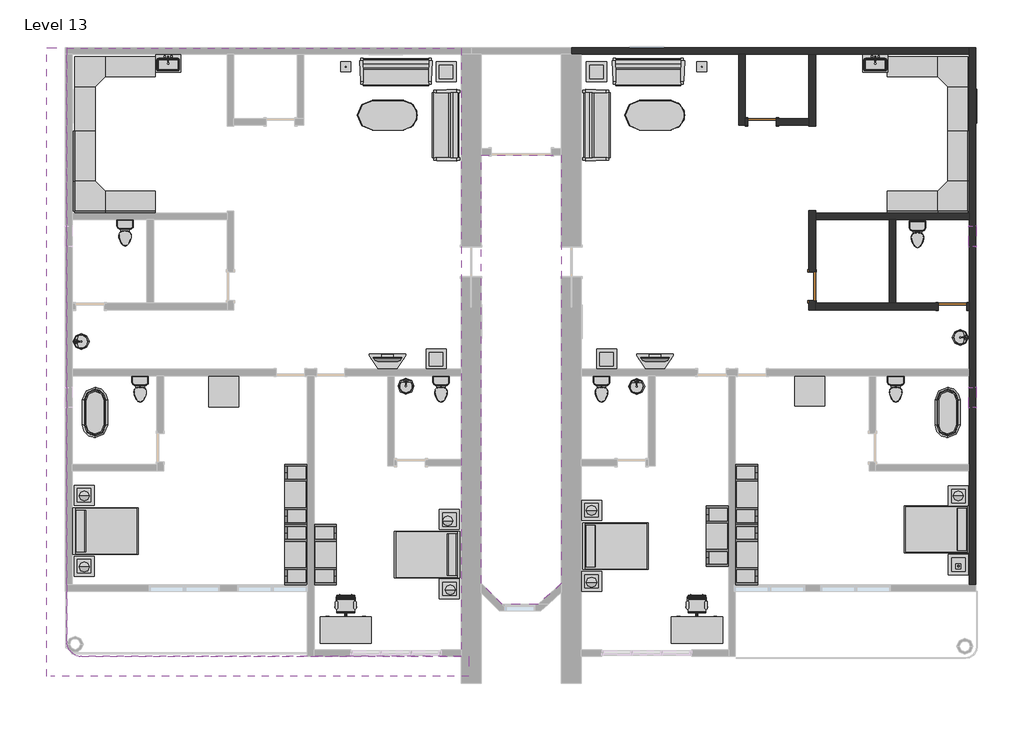
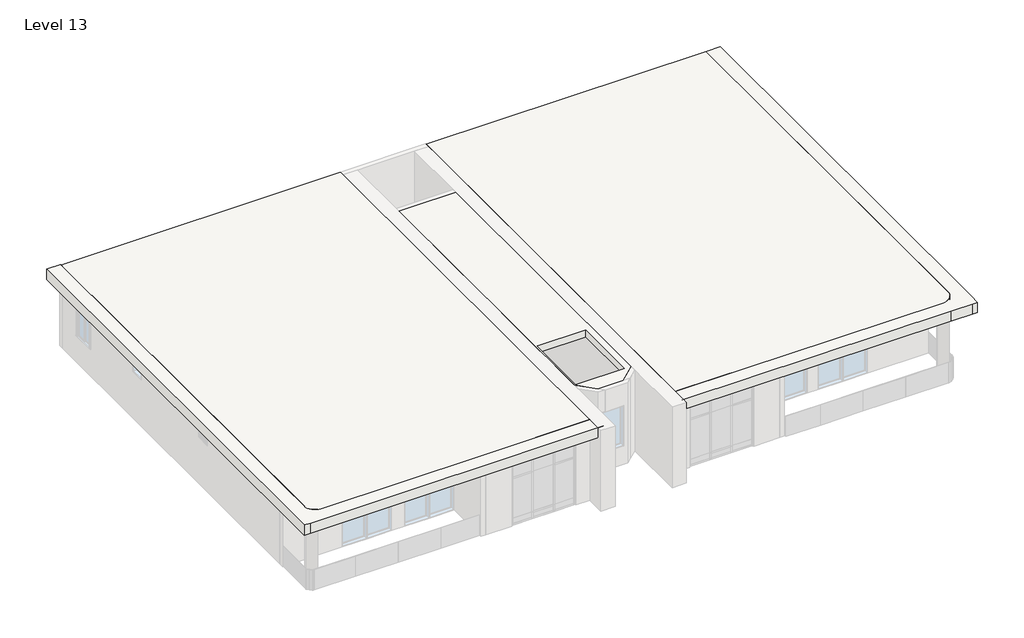
# One storey, part 3 of 3: 42 furniture elements, 14 flow terminals, 10 light fixtures, 9 walls, 3 doors, 3 slabs, 3 windows.
"""IFC4 building model written with IfcOpenShell, lengths in millimetres."""

from ifc_helpers import new_model, si_unit, point, frame, frame_2d, origin, place, context, project, spatial, polyline, circle_curve, trimmed, segment, composite_curve, outline, extrude, faceted_brep, transform, mapped, element, save
from components import door_2703ae13, door_10fd3a06, flow_terminal_38af2918, flow_terminal_d49f872f, toilet_domestic_3d_toilet_domestic_3d_f7549cf7, toilet_domestic_3d_toilet_domestic_3d_183bbd19, flow_terminal_b374fae2, furniture_07436f11, furniture_096e7f55, chair_task_arms_chair_task_arms_fa5a08ef, furniture_072f6425, furniture_cf0b6580, furniture_aff9b2fb, furniture_56245f3a, tv_stand_tv_stand_6ce107e5, furniture_b5c51a22, furniture_2c34a4f9, furniture_4d44e21c, furniture_45e3acac, light_fixture_100w_120v_8564026f, table_lamp_hemispheric_60w_120v_02721d88, window_0038ecf3, window_54100e87

model = new_model("IFC4")

# Units and contexts
model_context = context("Model", 3, world=origin())
ifc_project = project(units=[si_unit("LENGTHUNIT", "METRE", prefix="MILLI")], contexts=[model_context])

# Site, building, storey
site = spatial("IfcSite", under=ifc_project)
building = spatial("IfcBuilding", under=site)
storey = spatial("IfcBuildingStorey", under=building, Name="Level 13", Elevation=43891.2)

# Doors
placement = place(None, origin())
door_shape = door_2703ae13(model_context)
element("IfcDoor", 1, ObjectType="Door-Single-Panel.0001 : 34\" x 80\"", at=placement, inside=storey, context=model_context, shape_type="MappedRepresentation", body=[
    mapped(door_shape, transform((2522.0012296, 9464.0758558, 43891.2), x_axis=(-1.0, 0.0, 0.0), y_axis=(0.0, -1.0, 0.0), z_axis=(0.0, 0.0, 1.0))),
])
door_2_shape = door_10fd3a06(model_context)
element("IfcDoor", 2, ObjectType="Door-Single-Panel.0001 : 34\" x 80\"", at=placement, inside=storey, context=model_context, shape_type="MappedRepresentation", body=[
    mapped(door_2_shape, transform((8313.2012296, 3850.6758558, 43891.2), x_axis=(1.0, 0.0, 0.0), y_axis=(0.0, 1.0, 0.0), z_axis=(0.0, 0.0, 1.0))),
])
element("IfcDoor", 3, ObjectType="Door-Single-Panel.0001 : 34\" x 80\"", at=placement, inside=storey, context=model_context, shape_type="MappedRepresentation", body=[
    mapped(door_2_shape, transform((4046.0012296, 4460.2758558, 43891.2), x_axis=(0.0, -1.0, 0.0), y_axis=(1.0, 0.0, 0.0), z_axis=(0.0, 0.0, 1.0))),
])

# Flow terminals
flow_terminal_shape = flow_terminal_38af2918(model_context)
element("IfcFlowTerminal", 4, ObjectType="Sink Kitchen-Single : 30\" x 21\"", at=placement, inside=storey, context=model_context, shape_type="MappedRepresentation", body=[
    mapped(flow_terminal_shape, transform((-15540.388011, 11239.7304546, 43891.2), x_axis=(1.0, 0.0, 0.0), y_axis=(0.0, 1.0, 0.0), z_axis=(0.0, 0.0, 1.0))),
])
element("IfcFlowTerminal", 5, ObjectType="Sink Kitchen-Single : 30\" x 21\"", at=placement, inside=storey, context=model_context, shape_type="MappedRepresentation", body=[
    mapped(flow_terminal_shape, transform((5948.011989, 11239.7304546, 43891.2), x_axis=(1.0, 0.0, 0.0), y_axis=(0.0, 1.0, 0.0), z_axis=(0.0, 0.0, 1.0))),
])
flow_terminal_2_shape = flow_terminal_d49f872f(model_context)
element("IfcFlowTerminal", 6, ObjectType="Sink Vanity-Round : 19\" x 19\"", at=placement, inside=storey, context=model_context, shape_type="MappedRepresentation", body=[
    mapped(flow_terminal_2_shape, transform((-18084.6070794, 2687.2241152, 43891.2), x_axis=(0.0, 1.0, 0.0), y_axis=(-1.0, 0.0, 0.0), z_axis=(0.0, 0.0, 1.0))),
])
element("IfcFlowTerminal", 7, ObjectType="Sink Vanity-Round : 19\" x 19\"", at=placement, inside=storey, context=model_context, shape_type="MappedRepresentation", body=[
    mapped(flow_terminal_2_shape, transform((8462.2249463, 3007.5275963, 43891.2), x_axis=(0.0, -1.0, 0.0), y_axis=(1.0, 0.0, 0.0), z_axis=(0.0, 0.0, 1.0))),
])
element("IfcFlowTerminal", 8, ObjectType="Sink Vanity-Round : 19\" x 19\"", at=placement, inside=storey, context=model_context, shape_type="MappedRepresentation", body=[
    mapped(flow_terminal_2_shape, transform((-8395.050511, 1341.8921141, 43891.2), x_axis=(1.0, 0.0, 0.0), y_axis=(0.0, 1.0, 0.0), z_axis=(0.0, 0.0, 1.0))),
])
element("IfcFlowTerminal", 9, ObjectType="Sink Vanity-Round : 19\" x 19\"", at=placement, inside=storey, context=model_context, shape_type="MappedRepresentation", body=[
    mapped(flow_terminal_2_shape, transform((-1384.650511, 1331.0855344, 43891.2), x_axis=(1.0, 0.0, 0.0), y_axis=(0.0, 1.0, 0.0), z_axis=(0.0, 0.0, 1.0))),
])
toilet_domestic_3d_toilet_domestic_3d_shape = toilet_domestic_3d_toilet_domestic_3d_f7549cf7(model_context)
toilet_domestic_3d_toilet_domestic_3d_2_shape = toilet_domestic_3d_toilet_domestic_3d_183bbd19(model_context)
element("IfcFlowTerminal", 10, ObjectType="Toilet-Domestic-3D : Toilet-Domestic-3D", at=placement, inside=storey, context=model_context, shape_type="MappedRepresentation", body=[
    mapped(toilet_domestic_3d_toilet_domestic_3d_shape, transform((6586.0012296, 1247.7798284, 43891.2), x_axis=(1.0, 0.0, 0.0), y_axis=(0.0, 1.0, 0.0), z_axis=(0.0, 0.0, 1.0))),
    mapped(toilet_domestic_3d_toilet_domestic_3d_2_shape, transform((6586.0012296, 1247.7798284, 43891.2), x_axis=(1.0, 0.0, 0.0), y_axis=(0.0, 1.0, 0.0), z_axis=(0.0, 0.0, 1.0))),
])
element("IfcFlowTerminal", 11, ObjectType="Toilet-Domestic-3D : Toilet-Domestic-3D", at=placement, inside=storey, context=model_context, shape_type="MappedRepresentation", body=[
    mapped(toilet_domestic_3d_toilet_domestic_3d_shape, transform((-2354.7987704, 1247.7798284, 43891.2), x_axis=(1.0, 0.0, 0.0), y_axis=(0.0, 1.0, 0.0), z_axis=(0.0, 0.0, 1.0))),
    mapped(toilet_domestic_3d_toilet_domestic_3d_2_shape, transform((-2354.7987704, 1247.7798284, 43891.2), x_axis=(1.0, 0.0, 0.0), y_axis=(0.0, 1.0, 0.0), z_axis=(0.0, 0.0, 1.0))),
])
element("IfcFlowTerminal", 12, ObjectType="Toilet-Domestic-3D : Toilet-Domestic-3D", at=placement, inside=storey, context=model_context, shape_type="MappedRepresentation", body=[
    mapped(toilet_domestic_3d_toilet_domestic_3d_shape, transform((-16375.5987704, 1247.7798284, 43891.2), x_axis=(1.0, 0.0, 0.0), y_axis=(0.0, 1.0, 0.0), z_axis=(0.0, 0.0, 1.0))),
    mapped(toilet_domestic_3d_toilet_domestic_3d_2_shape, transform((-16375.5987704, 1247.7798284, 43891.2), x_axis=(1.0, 0.0, 0.0), y_axis=(0.0, 1.0, 0.0), z_axis=(0.0, 0.0, 1.0))),
])
element("IfcFlowTerminal", 13, ObjectType="Toilet-Domestic-3D : Toilet-Domestic-3D", at=placement, inside=storey, context=model_context, shape_type="MappedRepresentation", body=[
    mapped(toilet_domestic_3d_toilet_domestic_3d_shape, transform((-16832.7987704, 5997.5798284, 43891.2), x_axis=(1.0, 0.0, 0.0), y_axis=(0.0, 1.0, 0.0), z_axis=(0.0, 0.0, 1.0))),
    mapped(toilet_domestic_3d_toilet_domestic_3d_2_shape, transform((-16832.7987704, 5997.5798284, 43891.2), x_axis=(1.0, 0.0, 0.0), y_axis=(0.0, 1.0, 0.0), z_axis=(0.0, 0.0, 1.0))),
])
element("IfcFlowTerminal", 14, ObjectType="Toilet-Domestic-3D : Toilet-Domestic-3D", at=placement, inside=storey, context=model_context, shape_type="MappedRepresentation", body=[
    mapped(toilet_domestic_3d_toilet_domestic_3d_shape, transform((7246.4012296, 5946.7798284, 43891.2), x_axis=(1.0, 0.0, 0.0), y_axis=(0.0, 1.0, 0.0), z_axis=(0.0, 0.0, 1.0))),
    mapped(toilet_domestic_3d_toilet_domestic_3d_2_shape, transform((7246.4012296, 5946.7798284, 43891.2), x_axis=(1.0, 0.0, 0.0), y_axis=(0.0, 1.0, 0.0), z_axis=(0.0, 0.0, 1.0))),
])
element("IfcFlowTerminal", 15, ObjectType="Toilet-Domestic-3D : Toilet-Domestic-3D", at=placement, inside=storey, context=model_context, shape_type="MappedRepresentation", body=[
    mapped(toilet_domestic_3d_toilet_domestic_3d_shape, transform((-7231.5987704, 1247.7798284, 43891.2), x_axis=(1.0, 0.0, 0.0), y_axis=(0.0, 1.0, 0.0), z_axis=(0.0, 0.0, 1.0))),
    mapped(toilet_domestic_3d_toilet_domestic_3d_2_shape, transform((-7231.5987704, 1247.7798284, 43891.2), x_axis=(1.0, 0.0, 0.0), y_axis=(0.0, 1.0, 0.0), z_axis=(0.0, 0.0, 1.0))),
])
flow_terminal_3_shape = flow_terminal_b374fae2(model_context)
element("IfcFlowTerminal", 16, ObjectType="Tub-Free Standing-3D : 30\" x 60\"", at=placement, inside=storey, context=model_context, shape_type="MappedRepresentation", body=[
    mapped(flow_terminal_3_shape, transform((-17747.1987704, 624.8758558, 43891.2), x_axis=(1.0, 0.0, 0.0), y_axis=(0.0, 1.0, 0.0), z_axis=(0.0, 0.0, 1.0))),
])
element("IfcFlowTerminal", 17, ObjectType="Tub-Free Standing-3D : 30\" x 60\"", at=placement, inside=storey, context=model_context, shape_type="MappedRepresentation", body=[
    mapped(flow_terminal_3_shape, transform((8160.8012296, 624.8758558, 43891.2), x_axis=(1.0, 0.0, 0.0), y_axis=(0.0, 1.0, 0.0), z_axis=(0.0, 0.0, 1.0))),
])

# Furniture
furniture_shape = furniture_07436f11(model_context)
element("IfcFurniture", 18, ObjectType="96\" x 96\"", at=placement, inside=storey, context=model_context, shape_type="MappedRepresentation", body=[
    mapped(furniture_shape, transform((-18275.8670182, 11991.0988634, 43891.2), x_axis=(1.0, 0.0, 0.0), y_axis=(0.0, 1.0, 0.0), z_axis=(0.0, 0.0, 1.0))),
])
element("IfcFurniture", 19, ObjectType="96\" x 96\"", at=placement, inside=storey, context=model_context, shape_type="MappedRepresentation", body=[
    mapped(furniture_shape, transform((9316.2242372, 11364.3441035, 43891.2), x_axis=(0.0, -1.0, 0.0), y_axis=(1.0, 0.0, 0.0), z_axis=(0.0, 0.0, 1.0))),
])
furniture_2_shape = furniture_096e7f55(model_context)
element("IfcFurniture", 20, ObjectType="Bed-Shaker : Double 56\" x 78\"", at=placement, inside=storey, context=model_context, shape_type="MappedRepresentation", body=[
    mapped(furniture_2_shape, transform((-18407.5987704, -2962.8741442, 43891.2), x_axis=(0.0, 1.0, 0.0), y_axis=(-1.0, 0.0, 0.0), z_axis=(0.0, 0.0, 1.0))),
])
element("IfcFurniture", 21, ObjectType="Bed-Shaker : Double 56\" x 78\"", at=placement, inside=storey, context=model_context, shape_type="MappedRepresentation", body=[
    mapped(furniture_2_shape, transform((-6672.7987704, -3712.1741442, 43891.2), x_axis=(0.0, -1.0, 0.0), y_axis=(1.0, 0.0, 0.0), z_axis=(0.0, 0.0, 1.0))),
])
element("IfcFurniture", 22, ObjectType="Bed-Shaker : Double 56\" x 78\"", at=placement, inside=storey, context=model_context, shape_type="MappedRepresentation", body=[
    mapped(furniture_2_shape, transform((-2913.5987704, -3420.0741442, 43891.2), x_axis=(0.0, 1.0, 0.0), y_axis=(-1.0, 0.0, 0.0), z_axis=(0.0, 0.0, 1.0))),
])
element("IfcFurniture", 23, ObjectType="Bed-Shaker : Double 56\" x 78\"", at=placement, inside=storey, context=model_context, shape_type="MappedRepresentation", body=[
    mapped(furniture_2_shape, transform((8821.2012296, -2950.1741442, 43891.2), x_axis=(0.0, -1.0, 0.0), y_axis=(1.0, 0.0, 0.0), z_axis=(0.0, 0.0, 1.0))),
])
chair_task_arms_chair_task_arms_shape = chair_task_arms_chair_task_arms_fa5a08ef(model_context)
element("IfcFurniture", 24, ObjectType="Chair-Task Arms : Chair-Task Arms", at=placement, inside=storey, context=model_context, shape_type="MappedRepresentation", body=[
    mapped(chair_task_arms_chair_task_arms_shape, transform((681.7920493, -5184.3566833, 43891.2), x_axis=(-1.0, 0.0, 0.0), y_axis=(0.0, -1.0, 0.0), z_axis=(0.0, 0.0, 1.0))),
])
element("IfcFurniture", 25, ObjectType="Chair-Task Arms : Chair-Task Arms", at=placement, inside=storey, context=model_context, shape_type="MappedRepresentation", body=[
    mapped(chair_task_arms_chair_task_arms_shape, transform((-9986.2079507, -5184.3566833, 43891.2), x_axis=(-1.0, 0.0, 0.0), y_axis=(0.0, -1.0, 0.0), z_axis=(0.0, 0.0, 1.0))),
])
furniture_3_shape = furniture_072f6425(model_context)
element("IfcFurniture", 26, ObjectType="Desk : 60\" x 30\"", at=placement, inside=storey, context=model_context, shape_type="MappedRepresentation", body=[
    mapped(furniture_3_shape, transform((-10889.1987704, -6371.702585, 43891.2), x_axis=(1.0, 0.0, 0.0), y_axis=(0.0, 1.0, 0.0), z_axis=(0.0, 0.0, 1.0))),
])
element("IfcFurniture", 27, ObjectType="Desk : 60\" x 30\"", at=placement, inside=storey, context=model_context, shape_type="MappedRepresentation", body=[
    mapped(furniture_3_shape, transform((-221.1987704, -6371.702585, 43891.2), x_axis=(1.0, 0.0, 0.0), y_axis=(0.0, 1.0, 0.0), z_axis=(0.0, 0.0, 1.0))),
])
furniture_4_shape = furniture_cf0b6580(model_context)
element("IfcFurniture", 28, ObjectType="Entertainment Center : 72\" x 72\" x 24\"", at=placement, inside=storey, context=model_context, shape_type="MappedRepresentation", body=[
    mapped(furniture_4_shape, transform((1607.6012296, -3134.3241442, 43891.2), x_axis=(0.0, -1.0, 0.0), y_axis=(1.0, 0.0, 0.0), z_axis=(0.0, 0.0, 1.0))),
])
element("IfcFurniture", 29, ObjectType="Entertainment Center : 72\" x 72\" x 24\"", at=placement, inside=storey, context=model_context, shape_type="MappedRepresentation", body=[
    mapped(furniture_4_shape, transform((1607.6012296, -3693.1241442, 43891.2), x_axis=(0.0, 1.0, 0.0), y_axis=(-1.0, 0.0, 0.0), z_axis=(0.0, 0.0, 1.0))),
])
element("IfcFurniture", 30, ObjectType="Entertainment Center : 72\" x 72\" x 24\"", at=placement, inside=storey, context=model_context, shape_type="MappedRepresentation", body=[
    mapped(furniture_4_shape, transform((1607.6012296, -1864.3241442, 43891.2), x_axis=(0.0, 1.0, 0.0), y_axis=(-1.0, 0.0, 0.0), z_axis=(0.0, 0.0, 1.0))),
])
element("IfcFurniture", 31, ObjectType="Entertainment Center : 72\" x 72\" x 24\"", at=placement, inside=storey, context=model_context, shape_type="MappedRepresentation", body=[
    mapped(furniture_4_shape, transform((-11193.9987704, -3693.1241442, 43891.2), x_axis=(0.0, -1.0, 0.0), y_axis=(1.0, 0.0, 0.0), z_axis=(0.0, 0.0, 1.0))),
])
element("IfcFurniture", 32, ObjectType="Entertainment Center : 72\" x 72\" x 24\"", at=placement, inside=storey, context=model_context, shape_type="MappedRepresentation", body=[
    mapped(furniture_4_shape, transform((-11193.9987704, -1864.3241442, 43891.2), x_axis=(0.0, -1.0, 0.0), y_axis=(1.0, 0.0, 0.0), z_axis=(0.0, 0.0, 1.0))),
])
element("IfcFurniture", 33, ObjectType="Entertainment Center : 72\" x 72\" x 24\"", at=placement, inside=storey, context=model_context, shape_type="MappedRepresentation", body=[
    mapped(furniture_4_shape, transform((-11193.9987704, -3693.1241442, 43891.2), x_axis=(0.0, 1.0, 0.0), y_axis=(-1.0, 0.0, 0.0), z_axis=(0.0, 0.0, 1.0))),
])
furniture_5_shape = furniture_aff9b2fb(model_context)
element("IfcFurniture", 34, ObjectType="Sofa-Pensi : 84\"", at=placement, inside=storey, context=model_context, shape_type="MappedRepresentation", body=[
    mapped(furniture_5_shape, transform((-8881.8050204, 10710.9660197, 43891.2), x_axis=(1.0, 0.0, 0.0), y_axis=(0.0, 1.0, 0.0), z_axis=(0.0, 0.0, 1.0))),
])
element("IfcFurniture", 35, ObjectType="Sofa-Pensi : 84\"", at=placement, inside=storey, context=model_context, shape_type="MappedRepresentation", body=[
    mapped(furniture_5_shape, transform((-7356.3086065, 9641.0821058, 43891.2), x_axis=(0.0, -1.0, 0.0), y_axis=(1.0, 0.0, 0.0), z_axis=(0.0, 0.0, 1.0))),
])
element("IfcFurniture", 36, ObjectType="Sofa-Pensi : 84\"", at=placement, inside=storey, context=model_context, shape_type="MappedRepresentation", body=[
    mapped(furniture_5_shape, transform((-2230.0889343, 9083.8696058, 43891.2), x_axis=(0.0, 1.0, 0.0), y_axis=(-1.0, 0.0, 0.0), z_axis=(0.0, 0.0, 1.0))),
])
element("IfcFurniture", 37, ObjectType="Sofa-Pensi : 84\"", at=placement, inside=storey, context=model_context, shape_type="MappedRepresentation", body=[
    mapped(furniture_5_shape, transform((-1211.0050204, 10710.9660197, 43891.2), x_axis=(1.0, 0.0, 0.0), y_axis=(0.0, 1.0, 0.0), z_axis=(0.0, 0.0, 1.0))),
])
furniture_6_shape = furniture_56245f3a(model_context)
element("IfcFurniture", 38, ObjectType="TV - Flat Screen : 32\"", at=placement, inside=storey, context=model_context, shape_type="MappedRepresentation", body=[
    mapped(furniture_6_shape, transform((-8861.1432846, 2232.8144794, 44805.6), x_axis=(-1.0, 0.0, 0.0), y_axis=(0.0, -1.0, 0.0), z_axis=(0.0, 0.0, 1.0))),
])
element("IfcFurniture", 39, ObjectType="TV - Flat Screen : 32\"", at=placement, inside=storey, context=model_context, shape_type="MappedRepresentation", body=[
    mapped(furniture_6_shape, transform((-733.1432846, 2232.8144794, 44805.6), x_axis=(-1.0, 0.0, 0.0), y_axis=(0.0, -1.0, 0.0), z_axis=(0.0, 0.0, 1.0))),
])
tv_stand_tv_stand_shape = tv_stand_tv_stand_6ce107e5(model_context)
element("IfcFurniture", 40, ObjectType="TV Stand : TV Stand", at=placement, inside=storey, context=model_context, shape_type="MappedRepresentation", body=[
    mapped(tv_stand_tv_stand_shape, transform((-8732.0107683, 1945.6758558, 43891.2), x_axis=(-1.0, 0.0, 0.0), y_axis=(0.0, -1.0, 0.0), z_axis=(0.0, 0.0, 1.0))),
])
element("IfcFurniture", 41, ObjectType="TV Stand : TV Stand", at=placement, inside=storey, context=model_context, shape_type="MappedRepresentation", body=[
    mapped(tv_stand_tv_stand_shape, transform((-604.0107683, 1945.6758558, 43891.2), x_axis=(-1.0, 0.0, 0.0), y_axis=(0.0, -1.0, 0.0), z_axis=(0.0, 0.0, 1.0))),
])
furniture_7_shape = furniture_b5c51a22(model_context)
element("IfcFurniture", 42, ObjectType="Table-Coffee : 24\" x 24\" x 24\"", at=placement, inside=storey, context=model_context, shape_type="MappedRepresentation", body=[
    mapped(furniture_7_shape, transform((-7097.4645371, 10892.864778, 43891.2), x_axis=(1.0, 0.0, 0.0), y_axis=(0.0, 1.0, 0.0), z_axis=(0.0, 0.0, 1.0))),
])
element("IfcFurniture", 43, ObjectType="Table-Coffee : 24\" x 24\" x 24\"", at=placement, inside=storey, context=model_context, shape_type="MappedRepresentation", body=[
    mapped(furniture_7_shape, transform((-2525.4645371, 10892.864778, 43891.2), x_axis=(1.0, 0.0, 0.0), y_axis=(0.0, 1.0, 0.0), z_axis=(0.0, 0.0, 1.0))),
])
element("IfcFurniture", 44, ObjectType="Table-Coffee : 24\" x 24\" x 24\"", at=placement, inside=storey, context=model_context, shape_type="MappedRepresentation", body=[
    mapped(furniture_7_shape, transform((-7402.2645371, 2155.264778, 43891.2), x_axis=(1.0, 0.0, 0.0), y_axis=(0.0, 1.0, 0.0), z_axis=(0.0, 0.0, 1.0))),
])
element("IfcFurniture", 45, ObjectType="Table-Coffee : 24\" x 24\" x 24\"", at=placement, inside=storey, context=model_context, shape_type="MappedRepresentation", body=[
    mapped(furniture_7_shape, transform((-2220.6645371, 2155.264778, 43891.2), x_axis=(1.0, 0.0, 0.0), y_axis=(0.0, 1.0, 0.0), z_axis=(0.0, 0.0, 1.0))),
])
element("IfcFurniture", 46, ObjectType="Table-Coffee : 24\" x 24\" x 24\"", at=placement, inside=storey, context=model_context, shape_type="MappedRepresentation", body=[
    mapped(furniture_7_shape, transform((-2677.8645371, -4601.135222, 43891.2), x_axis=(1.0, 0.0, 0.0), y_axis=(0.0, 1.0, 0.0), z_axis=(0.0, 0.0, 1.0))),
])
element("IfcFurniture", 47, ObjectType="Table-Coffee : 24\" x 24\" x 24\"", at=placement, inside=storey, context=model_context, shape_type="MappedRepresentation", body=[
    mapped(furniture_7_shape, transform((-18095.6645371, -4143.935222, 43891.2), x_axis=(1.0, 0.0, 0.0), y_axis=(0.0, 1.0, 0.0), z_axis=(0.0, 0.0, 1.0))),
])
element("IfcFurniture", 48, ObjectType="Table-Coffee : 24\" x 24\" x 24\"", at=placement, inside=storey, context=model_context, shape_type="MappedRepresentation", body=[
    mapped(furniture_7_shape, transform((-18095.6645371, -1984.935222, 43891.2), x_axis=(1.0, 0.0, 0.0), y_axis=(0.0, 1.0, 0.0), z_axis=(0.0, 0.0, 1.0))),
])
element("IfcFurniture", 49, ObjectType="Table-Coffee : 24\" x 24\" x 24\"", at=placement, inside=storey, context=model_context, shape_type="MappedRepresentation", body=[
    mapped(furniture_7_shape, transform((-2677.8645371, -2442.135222, 43891.2), x_axis=(1.0, 0.0, 0.0), y_axis=(0.0, 1.0, 0.0), z_axis=(0.0, 0.0, 1.0))),
])
element("IfcFurniture", 50, ObjectType="Table-Coffee : 24\" x 24\" x 24\"", at=placement, inside=storey, context=model_context, shape_type="MappedRepresentation", body=[
    mapped(furniture_7_shape, transform((8472.7354629, -4093.135222, 43891.2), x_axis=(1.0, 0.0, 0.0), y_axis=(0.0, 1.0, 0.0), z_axis=(0.0, 0.0, 1.0))),
])
element("IfcFurniture", 51, ObjectType="Table-Coffee : 24\" x 24\" x 24\"", at=placement, inside=storey, context=model_context, shape_type="MappedRepresentation", body=[
    mapped(furniture_7_shape, transform((8472.7354629, -2010.335222, 43891.2), x_axis=(1.0, 0.0, 0.0), y_axis=(0.0, 1.0, 0.0), z_axis=(0.0, 0.0, 1.0))),
])
element("IfcFurniture", 52, ObjectType="Table-Coffee : 24\" x 24\" x 24\"", at=placement, inside=storey, context=model_context, shape_type="MappedRepresentation", body=[
    mapped(furniture_7_shape, transform((-6995.8645371, -4832.0414601, 43891.2), x_axis=(1.0, 0.0, 0.0), y_axis=(0.0, 1.0, 0.0), z_axis=(0.0, 0.0, 1.0))),
])
element("IfcFurniture", 53, ObjectType="Table-Coffee : 24\" x 24\" x 24\"", at=placement, inside=storey, context=model_context, shape_type="MappedRepresentation", body=[
    mapped(furniture_7_shape, transform((-6995.8645371, -2723.8414601, 43891.2), x_axis=(1.0, 0.0, 0.0), y_axis=(0.0, 1.0, 0.0), z_axis=(0.0, 0.0, 1.0))),
])
furniture_8_shape = furniture_2c34a4f9(model_context)
element("IfcFurniture", 54, ObjectType="Table-Dining Oval : 36\" x 72\"", at=placement, inside=storey, context=model_context, shape_type="MappedRepresentation", body=[
    mapped(furniture_8_shape, transform((-8455.3790983, 10025.3742164, 43891.2), x_axis=(1.0, 0.0, 0.0), y_axis=(0.0, 1.0, 0.0), z_axis=(0.0, 0.0, 1.0))),
])
element("IfcFurniture", 55, ObjectType="Table-Dining Oval : 36\" x 72\"", at=placement, inside=storey, context=model_context, shape_type="MappedRepresentation", body=[
    mapped(furniture_8_shape, transform((-327.3790983, 10025.3742164, 43891.2), x_axis=(1.0, 0.0, 0.0), y_axis=(0.0, 1.0, 0.0), z_axis=(0.0, 0.0, 1.0))),
])
furniture_9_shape = furniture_4d44e21c(model_context)
element("IfcFurniture", 56, ObjectType="Table-Rectangular : 36\" x 36\"", at=placement, inside=storey, context=model_context, shape_type="MappedRepresentation", body=[
    mapped(furniture_9_shape, transform((-13835.5987704, 1259.8758558, 43891.2), x_axis=(1.0, 0.0, 0.0), y_axis=(0.0, 1.0, 0.0), z_axis=(0.0, 0.0, 1.0))),
])
element("IfcFurniture", 57, ObjectType="Table-Rectangular : 36\" x 36\"", at=placement, inside=storey, context=model_context, shape_type="MappedRepresentation", body=[
    mapped(furniture_9_shape, transform((3969.8012296, 1285.2758558, 43891.2), x_axis=(1.0, 0.0, 0.0), y_axis=(0.0, 1.0, 0.0), z_axis=(0.0, 0.0, 1.0))),
])
furniture_10_shape = furniture_45e3acac(model_context)
element("IfcFurniture", 58, ObjectType="Work Station Cubicle : 96\" x 96\"", at=placement, inside=storey, context=model_context, shape_type="MappedRepresentation", body=[
    mapped(furniture_10_shape, transform((-18902.621778, 6827.207608, 43891.2), x_axis=(0.0, 1.0, 0.0), y_axis=(-1.0, 0.0, 0.0), z_axis=(0.0, 0.0, 1.0))),
])
element("IfcFurniture", 59, ObjectType="Work Station Cubicle : 96\" x 96\"", at=placement, inside=storey, context=model_context, shape_type="MappedRepresentation", body=[
    mapped(furniture_10_shape, transform((8689.4694774, 6200.4528481, 43891.2), x_axis=(-1.0, 0.0, 0.0), y_axis=(0.0, -1.0, 0.0), z_axis=(0.0, 0.0, 1.0))),
])

# Light fixtures
light_fixture_100w_120v_shape = light_fixture_100w_120v_8564026f(model_context)
element("IfcLightFixture", 60, ObjectType="100W - 120V", at=placement, inside=storey, context=model_context, shape_type="MappedRepresentation", body=[
    mapped(light_fixture_100w_120v_shape, transform((-10127.1987704, 11140.4758558, 43891.2), x_axis=(1.0, 0.0, 0.0), y_axis=(0.0, 1.0, 0.0), z_axis=(0.0, 0.0, 1.0))),
])
element("IfcLightFixture", 61, ObjectType="100W - 120V", at=placement, inside=storey, context=model_context, shape_type="MappedRepresentation", body=[
    mapped(light_fixture_100w_120v_shape, transform((693.2012296, 11140.4758558, 43891.2), x_axis=(1.0, 0.0, 0.0), y_axis=(0.0, 1.0, 0.0), z_axis=(0.0, 0.0, 1.0))),
])
table_lamp_hemispheric_60w_120v_shape = table_lamp_hemispheric_60w_120v_02721d88(model_context)
element("IfcLightFixture", 62, ObjectType="Table Lamp - Hemispheric : 60W - 120V", at=placement, inside=storey, context=model_context, shape_type="MappedRepresentation", body=[
    mapped(table_lamp_hemispheric_60w_120v_shape, transform((-18077.3987704, -1915.1241442, 44500.8), x_axis=(1.0, 0.0, 0.0), y_axis=(0.0, 1.0, 0.0), z_axis=(0.0, 0.0, 1.0))),
])
element("IfcLightFixture", 63, ObjectType="Table Lamp - Hemispheric : 60W - 120V", at=placement, inside=storey, context=model_context, shape_type="MappedRepresentation", body=[
    mapped(table_lamp_hemispheric_60w_120v_shape, transform((-7028.3987704, -2666.7303823, 44500.8), x_axis=(1.0, 0.0, 0.0), y_axis=(0.0, 1.0, 0.0), z_axis=(0.0, 0.0, 1.0))),
])
element("IfcLightFixture", 64, ObjectType="Table Lamp - Hemispheric : 60W - 120V", at=placement, inside=storey, context=model_context, shape_type="MappedRepresentation", body=[
    mapped(table_lamp_hemispheric_60w_120v_shape, transform((-2659.5987704, -2346.9241442, 44500.8), x_axis=(1.0, 0.0, 0.0), y_axis=(0.0, 1.0, 0.0), z_axis=(0.0, 0.0, 1.0))),
])
element("IfcLightFixture", 65, ObjectType="Table Lamp - Hemispheric : 60W - 120V", at=placement, inside=storey, context=model_context, shape_type="MappedRepresentation", body=[
    mapped(table_lamp_hemispheric_60w_120v_shape, transform((8491.0012296, -4048.7241442, 44805.6), x_axis=(1.0, 0.0, 0.0), y_axis=(0.0, 1.0, 0.0), z_axis=(0.0, 0.0, 1.0))),
])
element("IfcLightFixture", 66, ObjectType="Table Lamp - Hemispheric : 60W - 120V", at=placement, inside=storey, context=model_context, shape_type="MappedRepresentation", body=[
    mapped(table_lamp_hemispheric_60w_120v_shape, transform((8491.0012296, -1915.1241442, 44500.8), x_axis=(1.0, 0.0, 0.0), y_axis=(0.0, 1.0, 0.0), z_axis=(0.0, 0.0, 1.0))),
])
element("IfcLightFixture", 67, ObjectType="Table Lamp - Hemispheric : 60W - 120V", at=placement, inside=storey, context=model_context, shape_type="MappedRepresentation", body=[
    mapped(table_lamp_hemispheric_60w_120v_shape, transform((-2659.5987704, -4531.3241442, 44500.8), x_axis=(1.0, 0.0, 0.0), y_axis=(0.0, 1.0, 0.0), z_axis=(0.0, 0.0, 1.0))),
])
element("IfcLightFixture", 68, ObjectType="Table Lamp - Hemispheric : 60W - 120V", at=placement, inside=storey, context=model_context, shape_type="MappedRepresentation", body=[
    mapped(table_lamp_hemispheric_60w_120v_shape, transform((-6952.1987704, -4762.2303823, 44500.8), x_axis=(1.0, 0.0, 0.0), y_axis=(0.0, 1.0, 0.0), z_axis=(0.0, 0.0, 1.0))),
])
element("IfcLightFixture", 69, ObjectType="Table Lamp - Hemispheric : 60W - 120V", at=placement, inside=storey, context=model_context, shape_type="MappedRepresentation", body=[
    mapped(table_lamp_hemispheric_60w_120v_shape, transform((-18077.3987704, -4074.1241442, 44500.8), x_axis=(1.0, 0.0, 0.0), y_axis=(0.0, 1.0, 0.0), z_axis=(0.0, 0.0, 1.0))),
])

# Slabs
element("IfcSlab", 70, ObjectType="Generic - 1.5' white 2", at=placement, inside=storey, context=model_context, shape_type="SweptSolid", body=[
    extrude(outline(composite_curve([segment(polyline([(9634.0012296, 11699.2758558), (9634.0012296, -6931.6241442), (9634.0012296, -7401.5241442), (9430.8012296, -7401.5241442), (8511.8043381, -7401.5241442), (-3015.1987704, -7401.5241442), (-3015.1987704, -6791.9241442), (8511.8043381, -6791.9241442)]), True, "CONTINUOUS"), segment(trimmed(circle_curve(frame_2d((8511.8043381, -6277.3874522)), 514.536692), [point((8511.8043381, -6791.9241442))], [point((9024.4012296, -6322.0241442))], True, "CARTESIAN"), True, "CONTINUOUS"), segment(polyline([(9024.4012296, -6322.0241442), (9024.4012296, 11699.2758558), (9634.0012296, 11699.2758558)]), True, "CONTINUOUS")], self_intersect=False)), frame((0.0, 0.0, 47091.6), z_axis=(0.0, 0.0, 1.0), x_axis=(1.0, 0.0, 0.0)), (0.0, 0.0, 1.0), 457.2),
    extrude(outline(composite_curve([segment(polyline([(-18610.7987704, 11724.6758558), (-18610.7987704, -6334.7241442)]), True, "CONTINUOUS"), segment(trimmed(circle_curve(frame_2d((-18153.5987704, -6334.7241442)), 457.2), [point((-18610.7987704, -6334.7241442))], [point((-18153.5987704, -6791.9241442))], True, "CARTESIAN"), True, "CONTINUOUS"), segment(polyline([(-18153.5987704, -6791.9241442), (-6393.3987704, -6791.9241442), (-6393.3987704, -7401.5241442), (-18966.3987704, -7401.5241442), (-19220.3987704, -7401.5241442), (-19220.3987704, 11724.6758558), (-18610.7987704, 11724.6758558)]), True, "CONTINUOUS")], self_intersect=False)), frame((0.0, 0.0, 47091.6), z_axis=(0.0, 0.0, 1.0), x_axis=(1.0, 0.0, 0.0)), (0.0, 0.0, 1.0), 457.2),
])
element("IfcSlab", 71, ObjectType="Generic - 12\" cream", at=placement, inside=storey, context=model_context, shape_type="SweptSolid", body=[
    extrude(outline(composite_curve([segment(polyline([(-6621.9987704, 11699.2758558), (-6621.9987704, -6791.9241442), (-11295.5987704, -6791.9241442), (-18153.5987704, -6791.9241442)]), True, "CONTINUOUS"), segment(trimmed(circle_curve(frame_2d((-18153.5987704, -6334.7241442)), 457.2), [point((-18153.5987704, -6791.9241442))], [point((-18610.7987704, -6334.7241442))], False, "CARTESIAN"), True, "CONTINUOUS"), segment(polyline([(-18610.7987704, -6334.7241442), (-18610.7987704, 11699.2758558), (-6621.9987704, 11699.2758558)]), True, "CONTINUOUS")], self_intersect=False)), frame((0.0, 0.0, 46939.2), z_axis=(0.0, 0.0, 1.0), x_axis=(1.0, 0.0, 0.0)), (0.0, 0.0, 1.0), 609.6),
    extrude(outline(composite_curve([segment(trimmed(circle_curve(frame_2d((8511.8043381, -6277.3874522)), 514.536692), [point((9024.4012296, -6322.0241442))], [point((8511.8043381, -6791.9241442))], False, "CARTESIAN"), True, "CONTINUOUS"), segment(polyline([(8511.8043381, -6791.9241442), (1709.2012296, -6791.9241442), (-2862.7987704, -6791.9241442), (-2964.3987704, -6791.9241442), (-2964.3987704, 11699.2758558), (9024.4012296, 11699.2758558), (9024.4012296, -6322.0241442)]), True, "CONTINUOUS")], self_intersect=False)), frame((0.0, 0.0, 46939.2), z_axis=(0.0, 0.0, 1.0), x_axis=(1.0, 0.0, 0.0)), (0.0, 0.0, 1.0), 609.6),
])
element("IfcSlab", 72, ObjectType="Generic - 12\" white", at=placement, inside=storey, context=model_context, shape_type="SweptSolid", body=[
    extrude(outline(polyline([(-3573.9987704, 8448.0758558), (-3573.9987704, -1691.5549149), (-3573.9987704, -4572.9908503), (-4280.7801413, -5203.302585), (-5374.5362318, -5203.302585), (-6012.3987704, -4565.4400463), (-6012.3987704, -1691.5549149), (-6012.3987704, 8448.0758558), (-3573.9987704, 8448.0758558)]), holes=[polyline([(-5940.8822214, -4528.8130548), (-5940.8822214, -4561.7549149), (-3858.0822214, -4561.7549149), (-3858.0822214, -1691.5549149), (-5940.8822214, -1691.5549149), (-5940.8822214, -4528.8130548)])]), frame((0.0, 0.0, 47244.0), z_axis=(0.0, 0.0, 1.0), x_axis=(1.0, 0.0, 0.0)), (0.0, 0.0, 1.0), 304.8),
])

# Walls
element("IfcWall", 73, ObjectType="Generic - 8\" cream", at=placement, inside=storey, context=model_context, shape_type="Brep", body=[
    faceted_brep([(8821.2012296, 11724.6758558, 43891.2), (8821.2012296, 11521.4758558, 43891.2), (8821.2012296, 6695.4758558, 43891.2), (8821.2012296, 6492.2758558, 43891.2), (8821.2012296, 3952.2758558, 43891.2), (8821.2012296, 3749.0758558, 43891.2), (8821.2012296, 1945.6758558, 43891.2), (8821.2012296, 1742.4758558, 43891.2), (8821.2012296, -949.9241442, 43891.2), (8821.2012296, -1153.1241442, 43891.2), (8821.2012296, -4607.5241442, 43891.2), (8821.2012296, -4607.5241442, 46939.2), (8821.2012296, -1153.1241442, 46939.2), (8821.2012296, -949.9241442, 46939.2), (8821.2012296, 1742.4758558, 46939.2), (8821.2012296, 1945.6758558, 46939.2), (8821.2012296, 3749.0758558, 46939.2), (8821.2012296, 3952.2758558, 46939.2), (8821.2012296, 6492.2758558, 46939.2), (8821.2012296, 6695.4758558, 46939.2), (8821.2012296, 11521.4758558, 46939.2), (8821.2012296, 11724.6758558, 46939.2), (8821.2012296, 10403.8758558, 45110.4), (8821.2012296, 10403.8758558, 46329.6), (8821.2012296, 9489.4758558, 46329.6), (8821.2012296, 9489.4758558, 45110.4), (8821.2012296, 777.2758558, 46634.4), (8821.2012296, 777.2758558, 46024.8), (8821.2012296, 1386.8758558, 46024.8), (8821.2012296, 1386.8758558, 46634.4), (8821.2012296, 6289.0758558, 46024.8), (8821.2012296, 6289.0758558, 46634.4), (8821.2012296, 5679.4758558, 46634.4), (8821.2012296, 5679.4758558, 46024.8), (9024.4012296, -4607.5241442, 43891.2), (9024.4012296, 11724.6758558, 43891.2), (9024.4012296, 11724.6758558, 46939.2), (9024.4012296, -4607.5241442, 46939.2), (9024.4012296, 10403.8758558, 46329.6), (9024.4012296, 10403.8758558, 45110.4), (9024.4012296, 9489.4758558, 45110.4), (9024.4012296, 9489.4758558, 46329.6), (9024.4012296, 777.2758558, 46024.8), (9024.4012296, 777.2758558, 46634.4), (9024.4012296, 1386.8758558, 46634.4), (9024.4012296, 1386.8758558, 46024.8), (9024.4012296, 6289.0758558, 46634.4), (9024.4012296, 6289.0758558, 46024.8), (9024.4012296, 5679.4758558, 46024.8), (9024.4012296, 5679.4758558, 46634.4)], [[[0, 1, 2, 3, 4, 5, 6, 7, 8, 9, 10, 11, 12, 13, 14, 15, 16, 17, 18, 19, 20, 21], [22, 23, 24, 25], [26, 27, 28, 29], [30, 31, 32, 33]], [[34, 35, 36, 37], [38, 39, 40, 41], [42, 43, 44, 45], [46, 47, 48, 49]], [[10, 9, 8, 7, 6, 5, 4, 3, 2, 1, 0, 35, 34]], [[21, 20, 19, 18, 17, 16, 15, 14, 13, 12, 11, 37, 36]], [[0, 21, 36, 35]], [[11, 10, 34, 37]], [[39, 38, 23, 22]], [[40, 39, 22, 25]], [[41, 40, 25, 24]], [[38, 41, 24, 23]], [[26, 43, 42, 27]], [[27, 42, 45, 28]], [[28, 45, 44, 29]], [[43, 26, 29, 44]], [[46, 31, 30, 47]], [[47, 30, 33, 48]], [[48, 33, 32, 49]], [[31, 46, 49, 32]]]),
])
element("IfcWall", 74, ObjectType="Generic - 8\" cream", at=placement, inside=storey, context=model_context, shape_type="Brep", body=[
    faceted_brep([(3944.4012296, 11521.4758558, 43891.2), (3944.4012296, 9565.6758558, 43891.2), (3944.4012296, 9362.4758558, 43891.2), (3944.4012296, 9337.0758558, 43891.2), (3944.4012296, 9337.0758558, 46939.2), (3944.4012296, 9362.4758558, 46939.2), (3944.4012296, 9565.6758558, 46939.2), (3944.4012296, 11521.4758558, 46939.2), (4147.6012296, 11521.4758558, 43891.2), (4147.6012296, 11521.4758558, 46939.2), (4147.6012296, 9337.0758558, 46939.2), (4147.6012296, 9337.0758558, 43891.2)], [[[0, 1, 2, 3, 4, 5, 6, 7]], [[8, 9, 10, 11]], [[3, 2, 1, 0, 8, 11]], [[4, 3, 11, 10]], [[7, 6, 5, 4, 10, 9]], [[0, 7, 9, 8]]]),
])
element("IfcWall", 75, ObjectType="Generic - 8\" cream", at=placement, inside=storey, context=model_context, shape_type="Brep", body=[
    faceted_brep([(4147.6012296, 6492.2758558, 43891.2), (6382.8012296, 6492.2758558, 43891.2), (6586.0012296, 6492.2758558, 43891.2), (8821.2012296, 6492.2758558, 43891.2), (8821.2012296, 6492.2758558, 46939.2), (6586.0012296, 6492.2758558, 46939.2), (6382.8012296, 6492.2758558, 46939.2), (4147.6012296, 6492.2758558, 46939.2), (4147.6012296, 6695.4758558, 43891.2), (4147.6012296, 6695.4758558, 46939.2), (8821.2012296, 6695.4758558, 46939.2), (8821.2012296, 6695.4758558, 43891.2)], [[[0, 1, 2, 3, 4, 5, 6, 7]], [[8, 9, 10, 11]], [[3, 2, 1, 0, 8, 11]], [[7, 6, 5, 4, 10, 9]], [[0, 7, 9, 8]], [[4, 3, 11, 10]]]),
])
element("IfcWall", 76, ObjectType="Generic - 8\" cream", at=placement, inside=storey, context=model_context, shape_type="Brep", body=[
    faceted_brep([(8821.2012296, 3749.0758558, 46939.2), (4147.6012296, 3749.0758558, 46939.2), (4147.6012296, 3749.0758558, 43891.2), (7881.4012296, 3749.0758558, 43891.2), (7881.4012296, 3749.0758558, 45923.2), (8745.0012296, 3749.0758558, 45923.2), (8745.0012296, 3749.0758558, 43891.2), (8821.2012296, 3749.0758558, 43891.2), (4147.6012296, 3952.2758558, 46939.2), (6382.8012296, 3952.2758558, 46939.2), (6586.0012296, 3952.2758558, 46939.2), (8821.2012296, 3952.2758558, 46939.2), (8821.2012296, 3952.2758558, 43891.2), (8745.0012296, 3952.2758558, 43891.2), (8745.0012296, 3952.2758558, 45923.2), (7881.4012296, 3952.2758558, 45923.2), (7881.4012296, 3952.2758558, 43891.2), (6586.0012296, 3952.2758558, 43891.2), (6382.8012296, 3952.2758558, 43891.2), (4147.6012296, 3952.2758558, 43891.2)], [[[0, 1, 2, 3, 4, 5, 6, 7]], [[8, 9, 10, 11, 12, 13, 14, 15, 16, 17, 18, 19]], [[2, 19, 18, 17, 16, 3]], [[12, 7, 6, 13]], [[1, 0, 11, 10, 9, 8]], [[2, 1, 8, 19]], [[0, 7, 12, 11]], [[5, 14, 13, 6]], [[14, 5, 4, 15]], [[15, 4, 3, 16]]]),
])
element("IfcWall", 77, ObjectType="Generic - 8\" cream", at=placement, inside=storey, context=model_context, shape_type="SweptSolid", body=[
    extrude(outline(polyline([(46939.2, 3944.4012296), (46939.2, 2014.0012296), (43891.2, 2014.0012296), (43891.2, 2090.2012296), (45923.2, 2090.2012296), (45923.2, 2953.8012296), (43891.2, 2953.8012296), (43891.2, 3944.4012296), (46939.2, 3944.4012296)])), frame((0.0, 9362.4758558, 0.0), z_axis=(0.0, 1.0, 0.0), x_axis=(0.0, 0.0, 1.0)), (0.0, 0.0, 1.0), 203.2),
])
element("IfcWall", 78, ObjectType="Generic - 8\" cream", at=placement, inside=storey, context=model_context, shape_type="SweptSolid", body=[
    extrude(outline(polyline([(6382.8012296, 3952.2758558), (6382.8012296, 6492.2758558), (6586.0012296, 6492.2758558), (6586.0012296, 3952.2758558), (6382.8012296, 3952.2758558)])), frame((0.0, 0.0, 43891.2), z_axis=(0.0, 0.0, 1.0), x_axis=(1.0, 0.0, 0.0)), (0.0, 0.0, 1.0), 3048.0),
])
element("IfcWall", 79, ObjectType="Generic - 8\" cream", at=placement, inside=storey, context=model_context, shape_type="Brep", body=[
    faceted_brep([(3944.4012296, 3749.0758558, 46939.2), (3944.4012296, 6771.6758558, 46939.2), (3944.4012296, 6771.6758558, 43891.2), (3944.4012296, 4892.0758558, 43891.2), (3944.4012296, 4892.0758558, 45923.2), (3944.4012296, 4028.4758558, 45923.2), (3944.4012296, 4028.4758558, 43891.2), (3944.4012296, 3749.0758558, 43891.2), (4147.6012296, 6771.6758558, 46939.2), (4147.6012296, 6695.4758558, 46939.2), (4147.6012296, 6492.2758558, 46939.2), (4147.6012296, 3952.2758558, 46939.2), (4147.6012296, 3749.0758558, 46939.2), (4147.6012296, 3749.0758558, 43891.2), (4147.6012296, 3952.2758558, 43891.2), (4147.6012296, 4028.4758558, 43891.2), (4147.6012296, 4028.4758558, 45923.2), (4147.6012296, 4892.0758558, 45923.2), (4147.6012296, 4892.0758558, 43891.2), (4147.6012296, 6492.2758558, 43891.2), (4147.6012296, 6695.4758558, 43891.2), (4147.6012296, 6771.6758558, 43891.2)], [[[0, 1, 2, 3, 4, 5, 6, 7]], [[8, 9, 10, 11, 12, 13, 14, 15, 16, 17, 18, 19, 20, 21]], [[2, 21, 20, 19, 18, 3]], [[13, 7, 6, 15, 14]], [[1, 0, 12, 11, 10, 9, 8]], [[2, 1, 8, 21]], [[0, 7, 13, 12]], [[5, 16, 15, 6]], [[16, 5, 4, 17]], [[17, 4, 3, 18]]]),
])
element("IfcWall", 80, ObjectType="Generic - 8\" cream", at=placement, inside=storey, context=model_context, shape_type="Brep", body=[
    faceted_brep([(-3269.1987704, 11521.4758558, 43891.2), (-2964.3987704, 11521.4758558, 43891.2), (1810.8012296, 11521.4758558, 43891.2), (2014.0012296, 11521.4758558, 43891.2), (3944.4012296, 11521.4758558, 43891.2), (4147.6012296, 11521.4758558, 43891.2), (8821.2012296, 11521.4758558, 43891.2), (8821.2012296, 11521.4758558, 46939.2), (4147.6012296, 11521.4758558, 46939.2), (3944.4012296, 11521.4758558, 46939.2), (2014.0012296, 11521.4758558, 46939.2), (1810.8012296, 11521.4758558, 46939.2), (-2964.3987704, 11521.4758558, 46939.2), (-3269.1987704, 11521.4758558, 46939.2), (-1440.3987704, 11521.4758558, 46329.6), (-525.9987704, 11521.4758558, 46329.6), (-525.9987704, 11521.4758558, 45110.4), (-1440.3987704, 11521.4758558, 45110.4), (-3269.1987704, 11724.6758558, 43891.2), (-3269.1987704, 11724.6758558, 46939.2), (-2964.3987704, 11724.6758558, 46939.2), (8821.2012296, 11724.6758558, 46939.2), (8821.2012296, 11724.6758558, 43891.2), (-1440.3987704, 11724.6758558, 46329.6), (-1440.3987704, 11724.6758558, 45110.4), (-525.9987704, 11724.6758558, 45110.4), (-525.9987704, 11724.6758558, 46329.6)], [[[0, 1, 2, 3, 4, 5, 6, 7, 8, 9, 10, 11, 12, 13], [14, 15, 16, 17]], [[18, 19, 20, 21, 22], [23, 24, 25, 26]], [[6, 5, 4, 3, 2, 1, 0, 18, 22]], [[13, 12, 11, 10, 9, 8, 7, 21, 20, 19]], [[0, 13, 19, 18]], [[7, 6, 22, 21]], [[23, 26, 15, 14]], [[26, 25, 16, 15]], [[25, 24, 17, 16]], [[24, 23, 14, 17]]]),
])
element("IfcWall", 81, ObjectType="Generic - 8\" white", at=placement, inside=storey, context=model_context, shape_type="Brep", body=[
    faceted_brep([(1810.8012296, 11521.4758558, 43891.2), (1810.8012296, 9362.4758558, 43891.2), (1810.8012296, 9362.4758558, 46939.2), (1810.8012296, 11521.4758558, 46939.2), (2014.0012296, 11521.4758558, 43891.2), (2014.0012296, 11521.4758558, 46939.2), (2014.0012296, 9565.6758558, 46939.2), (2014.0012296, 9362.4758558, 46939.2), (2014.0012296, 9362.4758558, 43891.2), (2014.0012296, 9565.6758558, 43891.2)], [[[0, 1, 2, 3]], [[4, 5, 6, 7, 8, 9]], [[1, 0, 4, 9, 8]], [[3, 2, 7, 6, 5]], [[0, 3, 5, 4]], [[2, 1, 8, 7]]]),
])

# Windows
window_shape = window_0038ecf3(model_context)
element("IfcWindow", 82, ObjectType="Louvers with Trim : 24\" x 24\"", at=placement, inside=storey, context=model_context, shape_type="MappedRepresentation", body=[
    mapped(window_shape, transform((8916.4512296, 5984.2758558, 45110.4), x_axis=(0.0, 1.0, 0.0), y_axis=(-1.0, 0.0, 0.0), z_axis=(0.0, 0.0, 1.0))),
])
element("IfcWindow", 83, ObjectType="Louvers with Trim : 24\" x 24\"", at=placement, inside=storey, context=model_context, shape_type="MappedRepresentation", body=[
    mapped(window_shape, transform((8929.1512296, 1082.0758558, 45110.4), x_axis=(0.0, -1.0, 0.0), y_axis=(1.0, 0.0, 0.0), z_axis=(0.0, 0.0, 1.0))),
])
window_2_shape = window_54100e87(model_context)
element("IfcWindow", 84, ObjectType="Slider with Trim : 36\" x 48\"", at=placement, inside=storey, context=model_context, shape_type="MappedRepresentation", body=[
    mapped(window_2_shape, transform((8922.8012296, 9946.6758558, 44196.0), x_axis=(0.0, 1.0, 0.0), y_axis=(-1.0, 0.0, 0.0), z_axis=(0.0, 0.0, 1.0))),
])

save(model, "model.ifc")

# Revit data of these elements
# Type "Door-Single-Panel.0001 : 34\" x 80\""
#   Type Mark = "9"
#   Construction Type Id = "DOOR"
#   Assembly Code = "C1020300"
#   Analytic Construction = "Wooden"
#   Thickness = 0' - 2"
#   Thermal Resistance (R) = 0.455703 (m²·K)/W
#   Swing Angle [instance default] = 90.00°
#   Heat Transfer Coefficient (U) = 2.19465 W/(m²·K)
#   Height = 6' - 8"
#   Trim Projection Ext = 0' - 1"
#   Trim Projection Int = 0' - 1"
#   Trim Width = 0' - 3"
#   Width = 2' - 10"
#   Panel Material = Wood - Birch - Solid Stained Light Low Gloss
#   Trim Material = Paint - Sienna
#   Visual Light Transmittance = 0
#   Solar Heat Gain Coefficient = 0
#   Function = (empty or 0)
#   Wall Closure = (empty or 0)
# Type "Sink Kitchen-Single : 30\" x 21\""
#   Assembly Code = "D2010410"
#   Counter Height = 3' - 0"
#   Depth = 1' - 9"
#   Width = 2' - 6"
#   Faucet Material = Steel, Polished
#   Sink Material = Steel, Polished
# Type "Sink Vanity-Round : 19\" x 19\""
#   Assembly Code = "D2010400"
#   Top Of Counter = 2' - 7"
#   Basin Material = Porcelain, Linen
#   Faucet Material = Steel, Polished
# Type "Toilet-Domestic-3D : Toilet-Domestic-3D"
#   Assembly Code = "D2010110"
#   Toilet - Bowl/Basin Material = Porcelain, Linen
#   Toilet - Seat Material = Laminate, Linen, Matte
# Type "Tub-Free Standing-3D : 30\" x 60\""
#   Assembly Code = "D2010110"
#   Height = 1' - 6"
#   Length = 5' - 0"
#   Width = 2' - 6"
#   Tub Material = Porcelain, Ivory
# Type "96\" x 96\""
#   Assembly Code = "E2020"
#   Desktop Height = 2' - 6"
#   Desktop1 Width = 2' - 0"
#   Desktop2 Width = 2' - 0"
#   Panel1 Length = 5' - 0"
#   Panel2 Length = 5' - 0"
#   Work Top Material = Laminate, Ivory, Matte
# Type "Bed-Shaker : Double 56\" x 78\""
#   Assembly Code = "E2020200"
#   Length = 6' - 6"
#   Width = 4' - 8"
#   Frame Material = Birch
#   Mattress Material = Linen, White
# Type "Chair-Task Arms : Chair-Task Arms"
#   Assembly Code = "E2020200"
#   Base Material = Plastic, Opaque Black
#   Caster Material = Plastic, Opaque Black
#   Seat/Back Material = Textile - Slate Blue
# Type "Desk : 60\" x 30\""
#   Assembly Code = "E2020200"
#   Depth = 2' - 6"
#   Height = 2' - 6"
#   Leg Height = 0' - 6"
#   Width = 5' - 0"
#   Body Material = Laminate, Ivory, Matte
#   Handle/Leg Material = Steel, Chrome Plated
#   Top Material = Cherry
# Type "Entertainment Center : 72\" x 72\" x 24\""
#   Assembly Code = "E2020200"
#   Center Width = 2' - 8"
#   Depth = 2' - 0"
#   Height = 6' - 0"
#   Width = 6' - 0"
#   Material = none
# Type "Sofa-Pensi : 84\""
#   Assembly Code = "E2020200"
#   Length = 7' - 0"
#   Frame Material = Cherry
#   Seat Material = Linen, Beige
#   Feet Material = Steel, Chrome Plated
# Type "TV - Flat Screen : 32\""
#   SinAng = 0' - 0.0193"
#   L = 2' - 3.79372"
#   H = 1' - 3.6354"
#   Thickness = 0' - 4.33071"
#   Diagonal = 2' - 7.88976"
#   CosAng = 0' - 0.03431"
#   Stand [instance default] = yes
# Type "TV Stand : TV Stand"
#   Depth = 1' - 6"
#   Width = 3' - 8"
#   Height = 1' - 7 1/2"
#   Finish = Melamine - Gray
# Type "Table-Coffee : 24\" x 24\" x 24\""
#   Assembly Code = "E2020200"
#   Height = 2' - 0"
#   Length = 2' - 0"
#   Width = 2' - 0"
#   Top Material = none
#   Frame Material = none
# Type "Table-Dining Oval : 36\" x 72\""
#   Assembly Code = "E2020200"
#   Length = 6' - 0"
#   Width = 3' - 0"
#   Base Material = Steel, Chrome Plated
#   Top Material = Glass - Clear, Grey
#   Description = (empty or 0)
# Type "Table-Rectangular : 36\" x 36\""
#   Assembly Code = "E2020200"
#   Height = 2' - 6"
#   Length = 3' - 0"
#   Width = 3' - 0"
#   Base Material = Birch
#   Top Material = Birch
# Type "Work Station Cubicle : 96\" x 96\""
#   Assembly Code = "E2020"
#   Desktop Height = 2' - 6"
#   Desktop1 Width = 2' - 0"
#   Desktop2 Width = 2' - 0"
#   Panel Height = 5' - 6"
#   Panel1 Length = 5' - 0"
#   Panel2 Length = 5' - 0"
#   Cube Panel Material = Textile - Light Gray
#   Work Top Material = Laminate, Ivory, Matte
# Type "100W - 120V"
#   Assembly Code = "D5020220"
#   Lamp = "A-19"
#   Wattage Comments = "100"
#   Wattage = 100 W
#   built-in parameter 1150110 = 1 (stored number, unit not read)
#   built-in parameter 1114217 = 1 (stored number, unit not read)
#   built-in parameter 1150109 = 1 (stored number, unit not read)
#   built-in parameter 1150113 = 1 (stored number, unit not read)
#   built-in parameter 1150115 = 1 (stored number, unit not read)
#   built-in parameter 1150105 = 139.261 (stored number, unit not read)
#   Light Source Symbol Size = 2' - 0"
#   built-in parameter 1150112 = 1 (stored number, unit not read)
#   built-in parameter 1150114 = 1 (stored number, unit not read)
#   built-in parameter 1150107 = 2800 (stored number, unit not read)
#   built-in parameter 1150106 = 1.39261 (stored number, unit not read)
#   built-in parameter 1150104 = 1.6258 (stored number, unit not read)
#   Ballast Voltage = 120 V
#   built-in parameter 1114218 = 1 (stored number, unit not read)
#   built-in parameter 1150133 = 10 (stored number, unit not read)
#   Lumens = 1750 lm
#   Apparent Load = 100 VA
#   built-in parameter 1150134 = 4
#   built-in parameter 1150137 = 1
#   Color Filter = 16777215
#   Ballast Number of Poles = 1
#   Shade = Glass, Frosted
#   Stand = Steel, Chrome Plated
#   Dimming Lamp Color Temperature Shift = (empty or 0)
# Type "Table Lamp - Hemispheric : 60W - 120V"
#   Assembly Code = "D5020220"
#   Lamp = "A-19"
#   Wattage = 60 W
#   built-in parameter 1150110 = 1 (stored number, unit not read)
#   built-in parameter 1114217 = 1 (stored number, unit not read)
#   built-in parameter 1150109 = 1 (stored number, unit not read)
#   built-in parameter 1150113 = 1 (stored number, unit not read)
#   built-in parameter 1150115 = 1 (stored number, unit not read)
#   built-in parameter 1150105 = 68.0387 (stored number, unit not read)
#   Light Source Symbol Size = 2' - 0"
#   built-in parameter 1150112 = 1 (stored number, unit not read)
#   built-in parameter 1150114 = 1 (stored number, unit not read)
#   built-in parameter 1150107 = 2800 (stored number, unit not read)
#   built-in parameter 1150106 = 0.680387 (stored number, unit not read)
#   built-in parameter 1150104 = 1.32387 (stored number, unit not read)
#   Ballast Voltage = 120 V
#   built-in parameter 1114218 = 1 (stored number, unit not read)
#   built-in parameter 1150133 = 10 (stored number, unit not read)
#   Lumens = 855 lm
#   Apparent Load = 60 VA
#   built-in parameter 1150134 = 4
#   built-in parameter 1150137 = 1
#   Color Filter = 16777215
#   Ballast Number of Poles = 1
#   Mount Material = Steel, Chrome Plated
#   Shade Material = Glass, Frosted
#   Base Material = Birch
#   Dimming Lamp Color Temperature Shift = (empty or 0)
#   Wattage Comments = ""
# Type "Generic - 1.5' white 2"
#   Assembly Code = "B1010"
#   Thickness = 1' - 6"
#   Function = 0
#   Layers, outside or top first: 1' - 6" "Door - Frame" (function 1)
# Type "Generic - 12\" cream"
#   Assembly Code = "B1010"
#   Thickness = 2' - 0"
#   Function = 0
#   Layers, outside or top first: 2' - 0" "Parking Stripe" (function 1)
# Type "Generic - 12\" white"
#   Assembly Code = "B1010"
#   Thickness = 1' - 0"
#   Function = 0
#   Layers, outside or top first: 1' - 0" "Door - Frame" (function 1)
# Type "Generic - 8\" cream"
#   Assembly Code = "B2010"
#   Width = 0' - 8"
#   Layers, outside or top first: 0' - 8" "Parking Stripe" (function 1)
# Type "Generic - 8\" white"
#   Assembly Code = "B2010"
#   Width = 0' - 8"
#   Layers, outside or top first: 0' - 8" "Door - Frame" (function 1)
# Type "Louvers with Trim : 24\" x 24\""
#   Type Mark = "27"
#   Construction Type Id = "GSP4R"
#   Assembly Code = "B20"
#   Analytic Construction = "1/8 in Pilkington single glazing"
#   Visual Light Transmittance = 0.9
#   Solar Heat Gain Coefficient = 0.78
#   Heat Transfer Coefficient (U) = 3.6886 W/(m²·K)
#   Default Sill Height = 3' - 0"
#   Trim Projection - Ext. = 0' - 0 1/2"
#   Trim Projection - Int. = 0' - 0 1/2"
#   Trim Width - Exterior = 0' - 1 1/2"
#   Trim Width - Interior = 0' - 1 1/2"
#   Width = 2' - 0"
#   Frame Material = Iron, Ductile
#   Louver Material = Glass
#   Trim Exterior Material = Glass
#   Trim Interior Material = Iron, Ductile
#   Wall Closure = (empty or 0)
# Type "Slider with Trim : 36\" x 48\""
#   Type Mark = "11"
#   Construction Type Id = "GSP4R"
#   Assembly Code = "B2020100"
#   Analytic Construction = "1/8 in Pilkington single glazing"
#   Visual Light Transmittance = 0.9
#   Solar Heat Gain Coefficient = 0.78
#   Heat Transfer Coefficient (U) = 3.6886 W/(m²·K)
#   Height = 4' - 0"
#   Default Sill Height = 3' - 0"
#   Trim Projection - Ext. = 0' - 0 3/4"
#   Trim Projection - Int. = 0' - 0 3/4"
#   Trim Width - Exterior = 0' - 3 1/2"
#   Trim Width - Interior = 0' - 3 1/2"
#   Width = 3' - 0"
#   Window Inset = 0' - 0 3/4"
#   Glass Pane Material = Glass
#   Sash Material = Iron, Ductile
#   Trim Exterior Material = Iron, Ductile
#   Trim Interior Material = Iron, Ductile
#   Wall Closure = (empty or 0)
# Elements 1, 2, 3 (IfcDoor, "Door-Single-Panel.0001 : 34\" x 80\"")
#   Swing Angle = 90.00°
#   Phase Created = New Construction
#   Materials on its faces: "Paint - Sienna", "Wood - Birch - Solid Stained Light Low Gloss"
# Element 4 (IfcFlowTerminal, "Sink Kitchen-Single : 30\" x 21\"")
#   Mark = "207"
#   Phase Created = New Construction
#   Materials on its faces: "Steel, Polished"
# Element 5 (IfcFlowTerminal, "Sink Kitchen-Single : 30\" x 21\"")
#   Mark = "208"
#   Phase Created = New Construction
#   Materials on its faces: "Steel, Polished"
# Element 6 (IfcFlowTerminal, "Sink Vanity-Round : 19\" x 19\"")
#   Mark = "211"
#   Phase Created = New Construction
#   Materials on its faces: "Porcelain, Linen", "Steel, Polished"
# Element 7 (IfcFlowTerminal, "Sink Vanity-Round : 19\" x 19\"")
#   Mark = "212"
#   Phase Created = New Construction
#   Materials on its faces: "Porcelain, Linen", "Steel, Polished"
# Element 8 (IfcFlowTerminal, "Sink Vanity-Round : 19\" x 19\"")
#   Mark = "219"
#   Phase Created = New Construction
#   Materials on its faces: "Porcelain, Linen", "Steel, Polished"
# Element 9 (IfcFlowTerminal, "Sink Vanity-Round : 19\" x 19\"")
#   Mark = "220"
#   Phase Created = New Construction
#   Materials on its faces: "Porcelain, Linen", "Steel, Polished"
# Element 10 (IfcFlowTerminal, "Toilet-Domestic-3D : Toilet-Domestic-3D")
#   Mark = "213"
#   Phase Created = New Construction
#   Materials on its faces: "Porcelain, Linen", "Laminate, Linen, Matte"
# Element 11 (IfcFlowTerminal, "Toilet-Domestic-3D : Toilet-Domestic-3D")
#   Mark = "214"
#   Phase Created = New Construction
#   Materials on its faces: "Porcelain, Linen", "Laminate, Linen, Matte"
# Element 12 (IfcFlowTerminal, "Toilet-Domestic-3D : Toilet-Domestic-3D")
#   Mark = "215"
#   Phase Created = New Construction
#   Materials on its faces: "Porcelain, Linen", "Laminate, Linen, Matte"
# Element 13 (IfcFlowTerminal, "Toilet-Domestic-3D : Toilet-Domestic-3D")
#   Mark = "216"
#   Phase Created = New Construction
#   Materials on its faces: "Porcelain, Linen", "Laminate, Linen, Matte"
# Element 14 (IfcFlowTerminal, "Toilet-Domestic-3D : Toilet-Domestic-3D")
#   Mark = "217"
#   Phase Created = New Construction
#   Materials on its faces: "Porcelain, Linen", "Laminate, Linen, Matte"
# Element 15 (IfcFlowTerminal, "Toilet-Domestic-3D : Toilet-Domestic-3D")
#   Mark = "218"
#   Phase Created = New Construction
#   Materials on its faces: "Porcelain, Linen", "Laminate, Linen, Matte"
# Element 16 (IfcFlowTerminal, "Tub-Free Standing-3D : 30\" x 60\"")
#   Mark = "205"
#   Phase Created = New Construction
#   Materials on its faces: "Porcelain, Ivory"
# Element 17 (IfcFlowTerminal, "Tub-Free Standing-3D : 30\" x 60\"")
#   Mark = "206"
#   Phase Created = New Construction
#   Materials on its faces: "Porcelain, Ivory"
# Elements 18, 19 (IfcFurniture, "96\" x 96\"")
#   Phase Created = New Construction
#   Materials on its faces: "Laminate, Ivory, Matte"
# Elements 20, 21, 22, 23 (IfcFurniture, "Bed-Shaker : Double 56\" x 78\"")
#   Phase Created = New Construction
#   Materials on its faces: "Birch", "Linen, White"
# Elements 24, 25 (IfcFurniture, "Chair-Task Arms : Chair-Task Arms")
#   Phase Created = New Construction
#   Materials on its faces: "Plastic, Opaque Black", "Textile - Slate Blue"
# Elements 26, 27 (IfcFurniture, "Desk : 60\" x 30\"")
#   Phase Created = New Construction
#   Materials on its faces: "Steel, Chrome Plated", "Laminate, Ivory, Matte", "Cherry"
# Elements 28, 29, 30, 31, 32, 33 (IfcFurniture, "Entertainment Center : 72\" x 72\" x 24\"")
#   Phase Created = New Construction
#   Materials on its faces: "Steel, Chrome Plated", "Glass - Clear, Grey"
# Elements 34, 35, 36, 37 (IfcFurniture, "Sofa-Pensi : 84\"")
#   Phase Created = New Construction
#   Materials on its faces: "Cherry", "Linen, Beige", "Steel, Chrome Plated"
